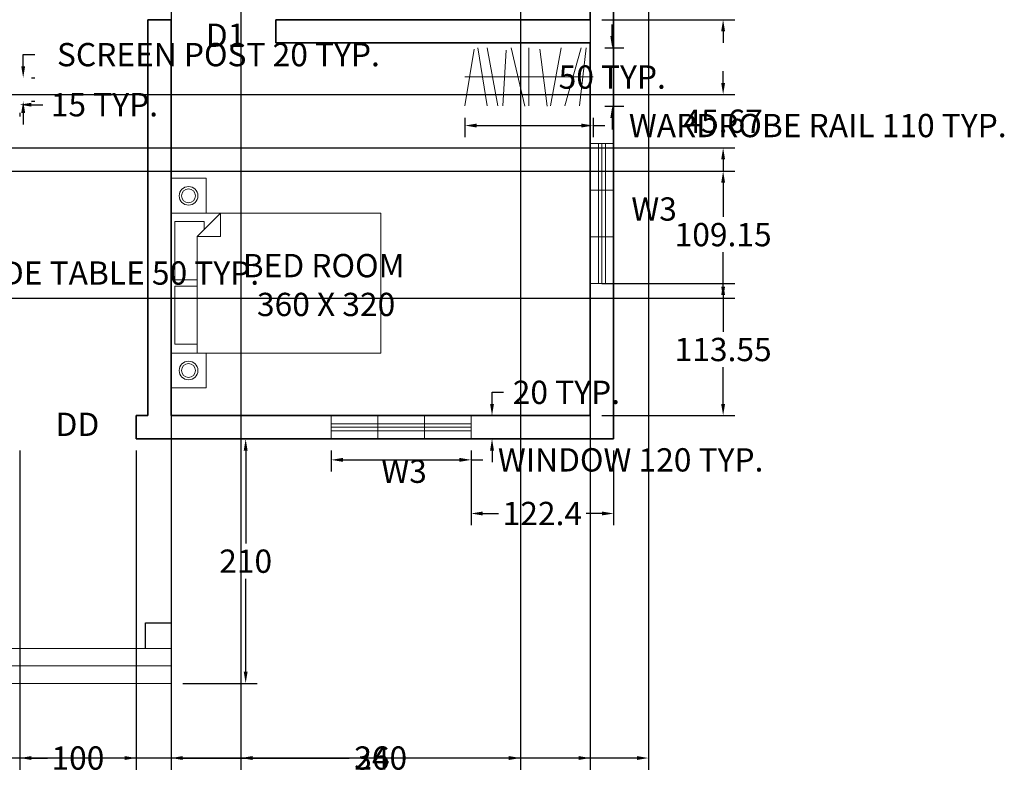
# Model space of a CAD drawing. Units: centimetres. Extents: x 543 to 2148, y 348 to 1642.
# Tile 3 of 4: x 1302 to 2148, y 348 to 995. Entities that reach past the tile are written whole.
import ezdxf

# ---------------------------------------------------------------- set-up
doc = ezdxf.new("R2010")
doc.units = ezdxf.units.CM
doc.header["$MEASUREMENT"] = 0
for name, color, linetype, lineweight in [('A-ANNO-DIMS', 2, 'Continuous', 18), ('A-ANNO-TEXT', 7, 'Continuous', 18), ('A-AREA-IDEN', 7, 'Continuous', 25), ('A-FLOR', 7, 'Continuous', 25), ('A-FLOR-CASE', 8, 'Continuous', 20), ('A-FLOR-STRS', 7, 'Continuous', 20), ('A-FURN', 8, 'Continuous', 18), ('A-GLAZ', 4, 'Continuous', 18), ('A-WALL', 7, 'Continuous', 35)]:
    doc.layers.add(name, color=color, linetype=linetype, lineweight=lineweight)
doc.styles.get("Standard").update_dxf_attribs({"font": 'arial.ttf'})
doc.dimstyles.get("Standard").update_dxf_attribs({"dimtxt": 20, "dimasz": 10, "dimexe": 10, "dimexo": 10, "dimgap": 5, "dimtad": 0, "dimtih": 1, "dimtoh": 1, "dimdec": 0, "dimzin": 0, "dimdsep": 46, "dimtxsty": 'Standard', "dimcen": 5, "dimadec": 0, "dimazin": 0, "dimtfac": 1, "dimtdec": 0, "dimtofl": 0, "dimtmove": 0, "dimatfit": 3, "dimfxl": 1, "dimtolj": 1, "dimtzin": 0, "dimarcsym": 0})

# ---------------------------------------------------------------- blocks, each defined once
blk = doc.blocks.new('BED-DOUBLE')
for p, q in [((42.36, 150), (22.36, 130)), ((42.36, 130), (42.36, 150)), ((22.36, 130), (22.36, 30)), ((22.36, 130), (42.36, 130)), ((3.32, 102.87), (3.32, 92.87)), ((3.32, 92.87), (22.36, 92.87)), ((3.32, 77.49), (3.32, 87.49)), ((3.32, 87.49), (22.36, 87.49))]:
    blk.add_line(p, q)
for points in [[(0, 150), (30, 150), (30, 180), (0, 180)], [(180, 150), (180, 30), (0, 30), (0, 150)], [(0, 0), (30, 0), (30, 30), (0, 30)]]:
    blk.add_lwpolyline(points, close=True)
for points in [[(3.32, 102.87), (3.32, 142.87), (28.32, 142.87), (28.32, 135.96)], [(22.36, 37.49), (3.32, 37.49), (3.32, 77.49)]]:
    blk.add_lwpolyline(points)
for centre, radius in [((15, 165), 8), ((15, 165), 6), ((15, 15), 8), ((15, 15), 6)]:
    blk.add_circle(centre, radius)
blk = doc.blocks.new('WARDROBE-RAIL')
for p, q in [((0, 0.31), (7.78, 49.18)), ((11.01, 50.31), (19.09, 0.31)), ((19.09, 50.31), (28.16, 0.3)), ((32.55, 0.31), (35.53, 48.25)), ((39.55, 50.31), (51.34, 0)), ((55, 0.31), (55, 50.31)), ((64.34, 49.01), (70.51, 0.27)), ((73.48, 0.31), (82.64, 50.31)), ((99.87, 50.31), (85.87, 0.31)), ((98.25, 0.31), (103.96, 50.31)), ((0, 25.31), (110, 25.31))]:
    blk.add_line(p, q)
blk = doc.blocks.new('WIN-1200')
for p, q in [((40, 20), (40, 0)), ((80, 20), (80, 0)), ((0, 13), (120, 13)), ((0, 10), (120, 10)), ((0, 7), (120, 7))]:
    blk.add_line(p, q)
blk.add_lwpolyline([(0, 20), (120, 20), (120, 0), (0, 0)], close=True)
blk = doc.blocks.new('*D13')
at = {"layer": 'A-ANNO-DIMS', "color": 0, "lineweight": -2, "transparency": 16777216}
for p, q in [((1569.73, 625.09), (1569.73, 607.09)), ((1689.73, 625.09), (1689.73, 607.09)), ((1579.73, 617.09), (1679.73, 617.09)), ((1689.73, 617.09), (1699.73, 617.09))]:
    blk.add_line(p, q, dxfattribs=at)
at = {"layer": 'A-ANNO-DIMS', "color": 0, "transparency": 16777216}
for points in [[(1579.73, 618.76), (1579.73, 615.43), (1569.73, 617.09)], [(1679.73, 618.76), (1679.73, 615.43), (1689.73, 617.09)]]:
    blk.add_solid(points, dxfattribs=at)
at = {"layer": 'Defpoints', "color": 0, "transparency": 16777216}
for p in [(1569.73, 635.09), (1689.73, 635.09), (1689.73, 617.09)]:
    blk.add_point(p, dxfattribs=at)
at = {"layer": 'A-ANNO-DIMS', "color": 0, "transparency": 16777216, "insert": (1826.77, 617.09), "char_height": 20, "attachment_point": 5}
blk.add_mtext('\\A1;WINDOW 120 TYP.', dxfattribs=at)
blk = doc.blocks.new('*D14')
at = {"layer": 'A-ANNO-DIMS', "color": 0, "lineweight": -2, "transparency": 16777216}
for p, q in [((1707.73, 665.09), (1707.73, 675.09)), ((1707.73, 675.09), (1717.73, 675.09)), ((1699.73, 655.09), (1717.73, 655.09)), ((1699.73, 635.09), (1717.73, 635.09)), ((1707.73, 625.09), (1707.73, 615.09))]:
    blk.add_line(p, q, dxfattribs=at)
at = {"layer": 'A-ANNO-DIMS', "color": 0, "transparency": 16777216}
for points in [[(1706.07, 665.09), (1709.4, 665.09), (1707.73, 655.09)], [(1706.07, 625.09), (1709.4, 625.09), (1707.73, 635.09)]]:
    blk.add_solid(points, dxfattribs=at)
at = {"layer": 'Defpoints', "color": 0, "transparency": 16777216}
for p in [(1689.73, 655.09), (1707.73, 655.09), (1689.73, 635.09)]:
    blk.add_point(p, dxfattribs=at)
at = {"layer": 'A-ANNO-DIMS', "color": 0, "transparency": 16777216, "insert": (1771.58, 675.09), "char_height": 20, "attachment_point": 5}
blk.add_mtext('\\A1;20 TYP.', dxfattribs=at)
blk = doc.blocks.new('*D17')
at = {"layer": 'A-ANNO-DIMS', "color": 0, "lineweight": -2, "transparency": 16777216}
for p, q in [((1305.14, 955.09), (1305.14, 965.09)), ((1305.14, 965.09), (1315.14, 965.09)), ((1312.14, 945.09), (1315.14, 945.09)), ((1312.14, 925.09), (1315.14, 925.09)), ((1305.14, 915.09), (1305.14, 905.09))]:
    blk.add_line(p, q, dxfattribs=at)
at = {"layer": 'A-ANNO-DIMS', "color": 0, "transparency": 16777216}
for points in [[(1303.47, 955.09), (1306.81, 955.09), (1305.14, 945.09)], [(1303.47, 915.09), (1306.81, 915.09), (1305.14, 925.09)]]:
    blk.add_solid(points, dxfattribs=at)
at = {"layer": 'Defpoints', "color": 0, "transparency": 16777216}
for p in [(1302.14, 945.09), (1305.14, 945.09), (1302.14, 925.09)]:
    blk.add_point(p, dxfattribs=at)
at = {"layer": 'A-ANNO-DIMS', "color": 0, "transparency": 16777216, "insert": (1472.79, 965.09), "char_height": 20, "attachment_point": 5}
blk.add_mtext('\\A1;SCREEN POST 20 TYP.', dxfattribs=at)
blk = doc.blocks.new('*D18')
at = {"layer": 'A-ANNO-DIMS', "color": 0, "lineweight": -2, "transparency": 16777216}
for p, q in [((1277.14, 922.09), (1267.14, 922.09)), ((1312.14, 922.09), (1322.14, 922.09)), ((1287.14, 915.09), (1287.14, 912.09)), ((1302.14, 915.09), (1302.14, 912.09))]:
    blk.add_line(p, q, dxfattribs=at)
at = {"layer": 'A-ANNO-DIMS', "color": 0, "transparency": 16777216}
for points in [[(1277.14, 923.76), (1277.14, 920.43), (1287.14, 922.09)], [(1312.14, 923.76), (1312.14, 920.43), (1302.14, 922.09)]]:
    blk.add_solid(points, dxfattribs=at)
at = {"layer": 'Defpoints', "color": 0, "transparency": 16777216}
for p in [(1287.14, 925.09), (1302.14, 925.09), (1302.14, 922.09)]:
    blk.add_point(p, dxfattribs=at)
at = {"layer": 'A-ANNO-DIMS', "color": 0, "transparency": 16777216, "insert": (1374.88, 922.09), "char_height": 20, "attachment_point": 5}
blk.add_mtext('\\A1;15 TYP.', dxfattribs=at)
blk = doc.blocks.new('*D25')
at = {"layer": 'A-ANNO-DIMS', "color": 0, "lineweight": -2, "transparency": 16777216}
for p, q in [((1684.48, 910.69), (1684.48, 894.19)), ((1794.48, 910.69), (1794.48, 894.19)), ((1694.48, 904.19), (1784.48, 904.19)), ((1794.48, 904.19), (1804.48, 904.19))]:
    blk.add_line(p, q, dxfattribs=at)
at = {"layer": 'A-ANNO-DIMS', "color": 0, "transparency": 16777216}
for points in [[(1694.48, 905.86), (1694.48, 902.52), (1684.48, 904.19)], [(1784.48, 905.86), (1784.48, 902.52), (1794.48, 904.19)]]:
    blk.add_solid(points, dxfattribs=at)
at = {"layer": 'Defpoints', "color": 0, "transparency": 16777216}
for p in [(1684.48, 920.69), (1794.48, 920.69), (1794.48, 904.19)]:
    blk.add_point(p, dxfattribs=at)
at = {"layer": 'A-ANNO-DIMS', "color": 0, "transparency": 16777216, "insert": (1987.43, 904.19), "char_height": 20, "attachment_point": 5}
blk.add_mtext('\\A1;WARDROBE RAIL 110 TYP.', dxfattribs=at)
blk = doc.blocks.new('*D26')
at = {"layer": 'A-ANNO-DIMS', "color": 0, "lineweight": -2, "transparency": 16777216}
for p, q in [((1810.98, 981), (1810.98, 991)), ((1804.48, 971), (1820.98, 971)), ((1804.48, 920.69), (1820.98, 920.69)), ((1810.98, 910.69), (1810.98, 900.69))]:
    blk.add_line(p, q, dxfattribs=at)
at = {"layer": 'A-ANNO-DIMS', "color": 0, "transparency": 16777216}
for points in [[(1809.32, 981), (1812.65, 981), (1810.98, 971)], [(1809.32, 910.69), (1812.65, 910.69), (1810.98, 920.69)]]:
    blk.add_solid(points, dxfattribs=at)
at = {"layer": 'Defpoints', "color": 0, "transparency": 16777216}
for p in [(1794.48, 971), (1810.98, 971), (1794.48, 920.69)]:
    blk.add_point(p, dxfattribs=at)
at = {"layer": 'A-ANNO-DIMS', "color": 0, "transparency": 16777216, "insert": (1810.98, 945.84), "char_height": 20, "attachment_point": 5}
blk.add_mtext('\\A1;50 TYP.', dxfattribs=at)
blk = doc.blocks.new('*D35')
at = {"layer": 'A-ANNO-DIMS', "color": 0, "lineweight": -2, "transparency": 16777216}
for p, q in [((1186.93, 775.04), (1186.93, 767.54)), ((1196.93, 777.54), (1226.93, 777.54)), ((1236.93, 777.54), (1246.93, 777.54)), ((1236.93, 775.04), (1236.93, 767.54))]:
    blk.add_line(p, q, dxfattribs=at)
at = {"layer": 'A-ANNO-DIMS', "color": 0, "transparency": 16777216}
for points in [[(1196.93, 779.21), (1196.93, 775.87), (1186.93, 777.54)], [(1226.93, 779.21), (1226.93, 775.87), (1236.93, 777.54)]]:
    blk.add_solid(points, dxfattribs=at)
at = {"layer": 'Defpoints', "color": 0, "transparency": 16777216}
for p in [(1186.93, 785.04), (1236.93, 785.04), (1236.93, 777.54)]:
    blk.add_point(p, dxfattribs=at)
at = {"layer": 'A-ANNO-DIMS', "color": 0, "transparency": 16777216, "insert": (1385.19, 777.54), "char_height": 20, "attachment_point": 5}
blk.add_mtext('\\A1;SIDE TABLE 50 TYP.', dxfattribs=at)
blk = doc.blocks.new('*D39')
at = {"layer": 'A-ANNO-DIMS', "color": 0, "lineweight": -2, "transparency": 16777216}
for p, q in [((1432.14, 1275.09), (1432.14, 351.04)), ((1792.14, 1275.09), (1792.14, 351.04)), ((1442.14, 361.04), (1585.09, 361.04)), ((1782.14, 361.04), (1639.19, 361.04))]:
    blk.add_line(p, q, dxfattribs=at)
at = {"layer": 'A-ANNO-DIMS', "color": 0, "transparency": 16777216}
for points in [[(1442.14, 362.71), (1442.14, 359.38), (1432.14, 361.04)], [(1782.14, 362.71), (1782.14, 359.38), (1792.14, 361.04)]]:
    blk.add_solid(points, dxfattribs=at)
at = {"layer": 'Defpoints', "color": 0, "transparency": 16777216}
for p in [(1432.14, 1285.09), (1792.14, 1285.09), (1792.14, 361.04)]:
    blk.add_point(p, dxfattribs=at)
at = {"layer": 'A-ANNO-DIMS', "color": 0, "transparency": 16777216, "insert": (1612.14, 361.04), "char_height": 20, "attachment_point": 5}
blk.add_mtext('\\A1;360', dxfattribs=at)
blk = doc.blocks.new('*D45')
at = {"layer": 'A-ANNO-DIMS', "color": 0, "lineweight": -2, "transparency": 16777216}
for p, q in [((1302.14, 625.09), (1302.14, 351.04)), ((1402.14, 625.09), (1402.14, 351.04)), ((1312.14, 361.04), (1326.02, 361.04)), ((1392.14, 361.04), (1378.26, 361.04))]:
    blk.add_line(p, q, dxfattribs=at)
at = {"layer": 'A-ANNO-DIMS', "color": 0, "transparency": 16777216}
for points in [[(1312.14, 362.71), (1312.14, 359.38), (1302.14, 361.04)], [(1392.14, 362.71), (1392.14, 359.38), (1402.14, 361.04)]]:
    blk.add_solid(points, dxfattribs=at)
at = {"layer": 'Defpoints', "color": 0, "transparency": 16777216}
for p in [(1302.14, 635.09), (1402.14, 635.09), (1402.14, 361.04)]:
    blk.add_point(p, dxfattribs=at)
at = {"layer": 'A-ANNO-DIMS', "color": 0, "transparency": 16777216, "insert": (1352.14, 361.04), "char_height": 20, "attachment_point": 5}
blk.add_mtext('\\A1;100', dxfattribs=at)
blk = doc.blocks.new('*D47')
at = {"layer": 'A-ANNO-DIMS', "color": 0, "lineweight": -2, "transparency": 16777216}
for p, q in [((1442.14, 635.09), (1506.19, 635.09)), ((1496.19, 625.09), (1496.19, 545.3)), ((1496.19, 435.09), (1496.19, 514.88)), ((1442.14, 425.09), (1506.19, 425.09))]:
    blk.add_line(p, q, dxfattribs=at)
at = {"layer": 'A-ANNO-DIMS', "color": 0, "transparency": 16777216}
for points in [[(1494.52, 625.09), (1497.86, 625.09), (1496.19, 635.09)], [(1494.52, 435.09), (1497.86, 435.09), (1496.19, 425.09)]]:
    blk.add_solid(points, dxfattribs=at)
at = {"layer": 'Defpoints', "color": 0, "transparency": 16777216}
for p in [(1432.14, 635.09), (1432.14, 425.09), (1496.19, 425.09)]:
    blk.add_point(p, dxfattribs=at)
at = {"layer": 'A-ANNO-DIMS', "color": 0, "transparency": 16777216, "insert": (1496.19, 530.09), "char_height": 20, "attachment_point": 5}
blk.add_mtext('\\A1;210', dxfattribs=at)
blk = doc.blocks.new('*D52')
at = {"layer": 'A-ANNO-DIMS', "color": 0, "lineweight": -2, "transparency": 16777216}
for p, q in [((1906.19, 1065.38), (1906.19, 1075.38)), ((1802.14, 1055.38), (1916.19, 1055.38)), ((1802.14, 995.09), (1916.19, 995.09)), ((1906.19, 985.09), (1906.19, 975.09))]:
    blk.add_line(p, q, dxfattribs=at)
at = {"layer": 'A-ANNO-DIMS', "color": 0, "transparency": 16777216}
for points in [[(1904.52, 1065.38), (1907.86, 1065.38), (1906.19, 1055.38)], [(1904.52, 985.09), (1907.86, 985.09), (1906.19, 995.09)]]:
    blk.add_solid(points, dxfattribs=at)
at = {"layer": 'Defpoints', "color": 0, "transparency": 16777216}
for p in [(1792.14, 1055.38), (1906.19, 1055.38), (1792.14, 995.09)]:
    blk.add_point(p, dxfattribs=at)
at = {"layer": 'A-ANNO-DIMS', "color": 0, "transparency": 16777216, "insert": (1906.19, 1025.24), "char_height": 20, "attachment_point": 5}
blk.add_mtext('\\A1;60.29', dxfattribs=at)
blk = doc.blocks.new('*D53')
at = {"layer": 'A-ANNO-DIMS', "color": 0, "lineweight": -2, "transparency": 16777216}
for p, q in [((1802.14, 768.64), (1916.19, 768.64)), ((1906.19, 758.64), (1906.19, 727.09)), ((1906.19, 665.09), (1906.19, 696.65)), ((1802.14, 655.09), (1916.19, 655.09))]:
    blk.add_line(p, q, dxfattribs=at)
at = {"layer": 'A-ANNO-DIMS', "color": 0, "transparency": 16777216}
for points in [[(1904.52, 758.64), (1907.86, 758.64), (1906.19, 768.64)], [(1904.52, 665.09), (1907.86, 665.09), (1906.19, 655.09)]]:
    blk.add_solid(points, dxfattribs=at)
at = {"layer": 'Defpoints', "color": 0, "transparency": 16777216}
for p in [(1792.14, 768.64), (1906.19, 768.64), (1792.14, 655.09)]:
    blk.add_point(p, dxfattribs=at)
at = {"layer": 'A-ANNO-DIMS', "color": 0, "transparency": 16777216, "insert": (1906.19, 711.87), "char_height": 20, "attachment_point": 5}
blk.add_mtext('\\A1;113.55', dxfattribs=at)
blk = doc.blocks.new('*D54')
at = {"layer": 'A-ANNO-DIMS', "color": 0, "lineweight": -2, "transparency": 16777216}
for p, q in [((1689.73, 625.09), (1689.73, 561.04)), ((1812.14, 625.09), (1812.14, 561.04)), ((1699.73, 571.04), (1713.17, 571.04)), ((1802.14, 571.04), (1788.7, 571.04))]:
    blk.add_line(p, q, dxfattribs=at)
at = {"layer": 'A-ANNO-DIMS', "color": 0, "transparency": 16777216}
for points in [[(1699.73, 572.71), (1699.73, 569.38), (1689.73, 571.04)], [(1802.14, 572.71), (1802.14, 569.38), (1812.14, 571.04)]]:
    blk.add_solid(points, dxfattribs=at)
at = {"layer": 'Defpoints', "color": 0, "transparency": 16777216}
for p in [(1689.73, 635.09), (1812.14, 635.09), (1689.73, 571.04)]:
    blk.add_point(p, dxfattribs=at)
at = {"layer": 'A-ANNO-DIMS', "color": 0, "transparency": 16777216, "insert": (1750.94, 571.04), "char_height": 20, "attachment_point": 5}
blk.add_mtext('\\A1;122.4', dxfattribs=at)
blk = doc.blocks.new('*D57')
at = {"layer": 'A-ANNO-DIMS', "color": 0, "lineweight": -2, "transparency": 16777216}
for p, q in [((667.14, 865.09), (1916.19, 865.09)), ((1906.19, 855.09), (1906.19, 825.73)), ((1906.19, 765.94), (1906.19, 795.31)), ((667.14, 755.94), (1916.19, 755.94))]:
    blk.add_line(p, q, dxfattribs=at)
at = {"layer": 'A-ANNO-DIMS', "color": 0, "transparency": 16777216}
for points in [[(1904.52, 855.09), (1907.86, 855.09), (1906.19, 865.09)], [(1904.52, 765.94), (1907.86, 765.94), (1906.19, 755.94)]]:
    blk.add_solid(points, dxfattribs=at)
at = {"layer": 'Defpoints', "color": 0, "transparency": 16777216}
for p in [(657.14, 865.09), (657.14, 755.94), (1906.19, 755.94)]:
    blk.add_point(p, dxfattribs=at)
at = {"layer": 'A-ANNO-DIMS', "color": 0, "transparency": 16777216, "insert": (1906.19, 810.52), "char_height": 20, "attachment_point": 5}
blk.add_mtext('\\A1;109.15', dxfattribs=at)
blk = doc.blocks.new('*D58')
at = {"layer": 'A-ANNO-DIMS', "color": 0, "lineweight": -2, "transparency": 16777216}
for p, q in [((1906.19, 940.76), (1906.19, 950.76)), ((717.14, 930.76), (1916.19, 930.76)), ((717.14, 885.09), (1916.19, 885.09)), ((1906.19, 875.09), (1906.19, 865.09))]:
    blk.add_line(p, q, dxfattribs=at)
at = {"layer": 'A-ANNO-DIMS', "color": 0, "transparency": 16777216}
for points in [[(1904.52, 940.76), (1907.86, 940.76), (1906.19, 930.76)], [(1904.52, 875.09), (1907.86, 875.09), (1906.19, 885.09)]]:
    blk.add_solid(points, dxfattribs=at)
at = {"layer": 'Defpoints', "color": 0, "transparency": 16777216}
for p in [(707.14, 930.76), (1906.19, 930.76), (707.14, 885.09)]:
    blk.add_point(p, dxfattribs=at)
at = {"layer": 'A-ANNO-DIMS', "color": 0, "transparency": 16777216, "insert": (1906.19, 907.92), "char_height": 20, "attachment_point": 5}
blk.add_mtext('\\A1;45.67', dxfattribs=at)
blk = doc.blocks.new('*D61')
at = {"layer": 'A-ANNO-DIMS', "color": 0, "lineweight": -2, "transparency": 16777216}
for p, q in [((1492.14, 1475.09), (1492.14, 351.04)), ((1732.14, 1475.09), (1732.14, 351.04)), ((1502.14, 361.04), (1584.91, 361.04)), ((1722.14, 361.04), (1639.37, 361.04))]:
    blk.add_line(p, q, dxfattribs=at)
at = {"layer": 'A-ANNO-DIMS', "color": 0, "transparency": 16777216}
for points in [[(1502.14, 362.71), (1502.14, 359.38), (1492.14, 361.04)], [(1722.14, 362.71), (1722.14, 359.38), (1732.14, 361.04)]]:
    blk.add_solid(points, dxfattribs=at)
at = {"layer": 'Defpoints', "color": 0, "transparency": 16777216}
for p in [(1492.14, 1485.09), (1732.14, 1485.09), (1732.14, 361.04)]:
    blk.add_point(p, dxfattribs=at)
at = {"layer": 'A-ANNO-DIMS', "color": 0, "transparency": 16777216, "insert": (1612.14, 361.04), "char_height": 20, "attachment_point": 5}
blk.add_mtext('\\A1;240', dxfattribs=at)
blk = doc.blocks.new('*D68')
at = {"layer": 'A-ANNO-DIMS', "color": 0, "lineweight": -2, "transparency": 16777216}
for p, q in [((1842.14, 1185.09), (1842.14, 351.04)), ((637.14, 415.09), (637.14, 351.04)), ((647.14, 361.04), (1205.64, 361.04)), ((1832.14, 361.04), (1273.64, 361.04))]:
    blk.add_line(p, q, dxfattribs=at)
at = {"layer": 'A-ANNO-DIMS', "color": 0, "transparency": 16777216}
for points in [[(647.14, 362.71), (647.14, 359.38), (637.14, 361.04)], [(1832.14, 362.71), (1832.14, 359.38), (1842.14, 361.04)]]:
    blk.add_solid(points, dxfattribs=at)
at = {"layer": 'Defpoints', "color": 0, "transparency": 16777216}
for p in [(1842.14, 1195.09), (637.14, 425.09), (1842.14, 361.04)]:
    blk.add_point(p, dxfattribs=at)
at = {"layer": 'A-ANNO-DIMS', "color": 0, "transparency": 16777216, "insert": (1239.64, 361.04), "char_height": 20, "attachment_point": 5}
blk.add_mtext('\\A1;1205', dxfattribs=at)

msp = doc.modelspace()

# ---------------------------------------------------------------- linework, layer by layer
at = {"layer": 'A-FLOR'}
for p, q in [((1432.141, 635.092), (1432.141, 485.092)), ((1410.141, 477.092), (1432.141, 477.092)), ((1410.141, 455.092), (1410.141, 477.092))]:
    msp.add_line(p, q, dxfattribs=at)
at = {"layer": 'A-FLOR-STRS'}
for p, q in [((1432.141, 425.092), (1432.141, 485.092)), ((1067.141, 455.092), (1432.141, 455.092)), ((1067.141, 440.092), (1432.141, 440.092)), ((1067.141, 425.092), (1432.141, 425.092))]:
    msp.add_line(p, q, dxfattribs=at)
at = {"layer": 'A-WALL'}
for p, q in [((1812.141, 635.092), (1812.141, 1195.092)), ((1792.141, 995.092), (1792.141, 1175.092)), ((1412.141, 995.092), (1412.141, 655.092)), ((1432.141, 995.092), (1412.141, 995.092)), ((1432.141, 975.092), (1432.141, 995.092)), ((1654.141, 995.092), (1522.141, 995.092)), ((1522.141, 975.092), (1522.141, 995.092)), ((1654.141, 995.092), (1664.141, 995.092)), ((1664.141, 995.092), (1792.141, 995.092)), ((1432.141, 975.092), (1432.141, 655.092)), ((1792.141, 975.092), (1522.141, 975.092)), ((1792.141, 655.092), (1792.141, 975.092)), ((1412.141, 655.092), (1402.141, 655.092)), ((1402.141, 655.092), (1402.141, 635.092)), ((1432.141, 655.092), (1792.141, 655.092)), ((1412.141, 635.092), (1402.141, 635.092)), ((1812.141, 635.092), (1412.141, 635.092))]:
    msp.add_line(p, q, dxfattribs=at)

# ---------------------------------------------------------------- block references
at = {"layer": 'A-FLOR-CASE'}
msp.add_blockref('WARDROBE-RAIL', (1684.485, 920.69), dxfattribs=at)
at = {"layer": 'A-FURN'}
msp.add_blockref('BED-DOUBLE', (1432.141, 678.857), dxfattribs=at)
at = {"layer": 'A-GLAZ', "rotation": 270.0000000000001}
msp.add_blockref('WIN-1200', (1792.141, 888.643), dxfattribs=at)
at = {"layer": 'A-GLAZ'}
msp.add_blockref('WIN-1200', (1569.733, 635.092), dxfattribs=at)

# ---------------------------------------------------------------- texts
at = {"layer": 'A-ANNO-TEXT', "char_height": 20, "attachment_point": 1}
for s, insert in [('D1', (1461.983, 991.705)), ('W3', (1827.357, 842.499)), ('DD', (1332.954, 657.597)), ('W3', (1612.651, 617.31))]:
    msp.add_mtext_dynamic_manual_height_columns(s, width=246.06417, gutter_width=1, heights=[0], dxfattribs=dict(at, insert=insert))
at = {"layer": 'A-AREA-IDEN', "insert": (1487.562, 793.897), "char_height": 20, "attachment_point": 1}
msp.add_mtext_dynamic_manual_height_columns(' BED ROOM\\P   360 X 320', width=246.06417, gutter_width=1, heights=[0], dxfattribs=at)

# ---------------------------------------------------------------- dimensions: what is measured, and where the dimension line sits
at = {"layer": 'A-ANNO-DIMS'}
for base, p1, p2, picture, middle in [((1732.141, 361.042), (1492.141, 1485.092), (1732.141, 1485.092), '*D61', (1612.141, 361.042)), ((1792.141, 361.042), (1432.141, 1285.092), (1792.141, 1285.092), '*D39', (1612.141, 361.042)), ((1842.141, 361.042), (637.141, 425.092), (1842.141, 1195.092), '*D68', (1239.641, 361.042)), ((1402.141, 361.042), (1302.141, 635.092), (1402.141, 635.092), '*D45', (1352.141, 361.042))]:
    dim = msp.add_linear_dim(base=base, p1=p1, p2=p2, dimstyle='Standard', override={"dimdec": 0, "dimlfac": 1, "dimrnd": 0, "dimzin": 0, "dimdsep": 46, "dimlunit": 2}, dxfattribs=at)
    dim.commit()
    dim.dimension.update_dxf_attribs({"geometry": picture, "text_midpoint": middle})
for base, p1, p2, angle, override, picture, middle in [((1906.191, 1055.382), (1792.141, 995.092), (1792.141, 1055.382), 90, {"dimdec": 2, "dimlfac": 1, "dimrnd": 0, "dimzin": 0, "dimdsep": 46, "dimlunit": 2}, '*D52', (1906.191, 1025.237)), ((1906.191, 930.758), (707.141, 885.092), (707.141, 930.758), 90, {"dimdec": 2, "dimlfac": 1, "dimrnd": 0, "dimzin": 0, "dimdsep": 46, "dimlunit": 2}, '*D58', (1906.191, 907.925)), ((1906.191, 755.945), (657.141, 865.092), (657.141, 755.945), 90, {"dimdec": 2, "dimlfac": 1, "dimrnd": 0, "dimzin": 0, "dimdsep": 46, "dimlunit": 2}, '*D57', (1906.191, 810.518)), ((1906.191, 768.643), (1792.141, 655.092), (1792.141, 768.643), 90, {"dimdec": 2, "dimlfac": 1, "dimrnd": 0, "dimzin": 0, "dimdsep": 46, "dimlunit": 2}, '*D53', (1906.191, 711.867)), ((1496.191, 425.092), (1432.141, 635.092), (1432.141, 425.092), 270, {"dimdec": 0, "dimlfac": 1, "dimrnd": 0, "dimzin": 0, "dimdsep": 46, "dimlunit": 2}, '*D47', (1496.191, 530.092)), ((1689.733, 571.042), (1812.141, 635.092), (1689.733, 635.092), 180, {"dimdec": 1, "dimlfac": 1, "dimrnd": 0, "dimzin": 0, "dimdsep": 46, "dimlunit": 2}, '*D54', (1750.937, 571.042))]:
    dim = msp.add_linear_dim(base=base, p1=p1, p2=p2, angle=angle, dimstyle='Standard', override=override, dxfattribs=at)
    dim.commit()
    dim.dimension.update_dxf_attribs({"geometry": picture, "text_midpoint": middle})
for base, p1, p2, text, picture, middle in [((1305.141, 945.092), (1302.141, 925.092), (1302.141, 945.092), 'SCREEN POST <> TYP.', '*D17', (1472.788, 965.092)), ((1810.985, 970.999), (1794.485, 920.69), (1794.485, 970.999), '<> TYP.', '*D26', (1810.985, 945.844)), ((1707.733, 655.092), (1689.733, 635.092), (1689.733, 655.092), '<> TYP.', '*D14', (1771.58, 675.092))]:
    dim = msp.add_linear_dim(base=base, p1=p1, p2=p2, angle=90, text=text, dimstyle='Standard', override={"dimdec": 0, "dimlfac": 1, "dimrnd": 0, "dimzin": 0, "dimdsep": 46, "dimlunit": 2}, dxfattribs=at)
    dim.commit()
    dim.dimension.update_dxf_attribs({"geometry": picture, "text_midpoint": middle})
for base, p1, p2, text, picture, middle in [((1794.485, 904.19), (1684.485, 920.69), (1794.485, 920.69), 'WARDROBE RAIL <> TYP.', '*D25', (1987.431, 904.19)), ((1302.141, 922.092), (1287.141, 925.092), (1302.141, 925.092), '<> TYP.', '*D18', (1374.876, 922.092)), ((1236.933, 777.539), (1186.933, 785.039), (1236.933, 785.039), 'SIDE TABLE <> TYP.', '*D35', (1385.187, 777.539)), ((1689.733, 617.092), (1569.733, 635.092), (1689.733, 635.092), 'WINDOW <> TYP.', '*D13', (1826.766, 617.092))]:
    dim = msp.add_linear_dim(base=base, p1=p1, p2=p2, text=text, dimstyle='Standard', override={"dimdec": 0, "dimlfac": 1, "dimrnd": 0, "dimzin": 0, "dimdsep": 46, "dimlunit": 2}, dxfattribs=at)
    dim.commit()
    dim.dimension.update_dxf_attribs({"geometry": picture, "text_midpoint": middle})

doc.saveas('drawing.dxf')
